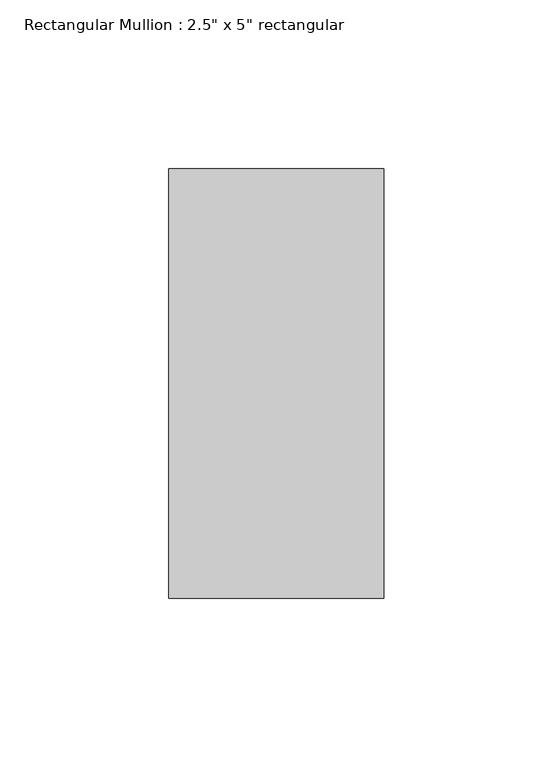
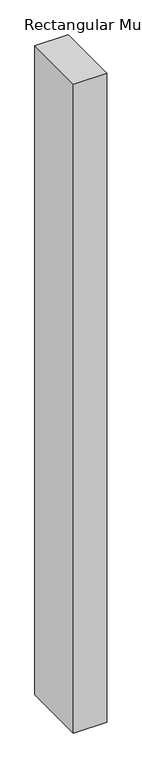
"""IFC4 building model written with IfcOpenShell, lengths in millimetres: member geometry."""

from ifc_helpers import new_model, si_unit, frame, origin, place, context, project, spatial, polyline, outline, extrude, source, transform, mapped, element, save


def member_1988fdfd(model_context):
    return source(origin(), model_context, "Body", "SweptSolid", [
        extrude(outline(polyline([(31.75, 63.5), (31.75, -63.5), (-31.75, -63.5), (-31.75, 63.5), (31.75, 63.5)])), frame((0.0, 0.0, -1308.1), z_axis=(0.0, 0.0, 1.0), x_axis=(1.0, 0.0, 0.0)), (0.0, 0.0, 1.0), 1308.1),
    ])


if __name__ == "__main__":
    model = new_model("IFC4")
    model_context = context("Model", 3, world=origin())
    ifc_project = project(units=[si_unit("LENGTHUNIT", "METRE", prefix="MILLI")], contexts=[model_context])
    site = spatial("IfcSite", under=ifc_project)
    building = spatial("IfcBuilding", under=site)
    placement = place(None, origin())
    member_shape = member_1988fdfd(model_context)
    element("IfcMember", 1, ObjectType="Rectangular Mullion : 2.5\" x 5\" rectangular", at=placement, inside=building, context=model_context, shape_type="MappedRepresentation", body=[
        mapped(member_shape, transform((0.0, 0.0, 0.0), x_axis=(1.0, 0.0, 0.0), y_axis=(0.0, 1.0, 0.0), z_axis=(0.0, 0.0, 1.0))),
    ])
    save(model, "model.ifc")

# Revit data of these elements
# Type "Rectangular Mullion : 2.5\" x 5\" rectangular"
#   built-in parameter 1007304 = 0.416667 (stored number, unit not read)
#   built-in parameter 1007301 = 0.104167 (stored number, unit not read)
#   built-in parameter 1007300 = 0.104167 (stored number, unit not read)
# Element 1 (IfcMember, "Rectangular Mullion : 2.5\" x 5\" rectangular")
#   Materials on its faces: "Aluminum"
# Materials
#   "Aluminum": class "Metal", colour RGB 247 247 247, transparency 0, Description = "Aluminum 6061", Cost = 0
